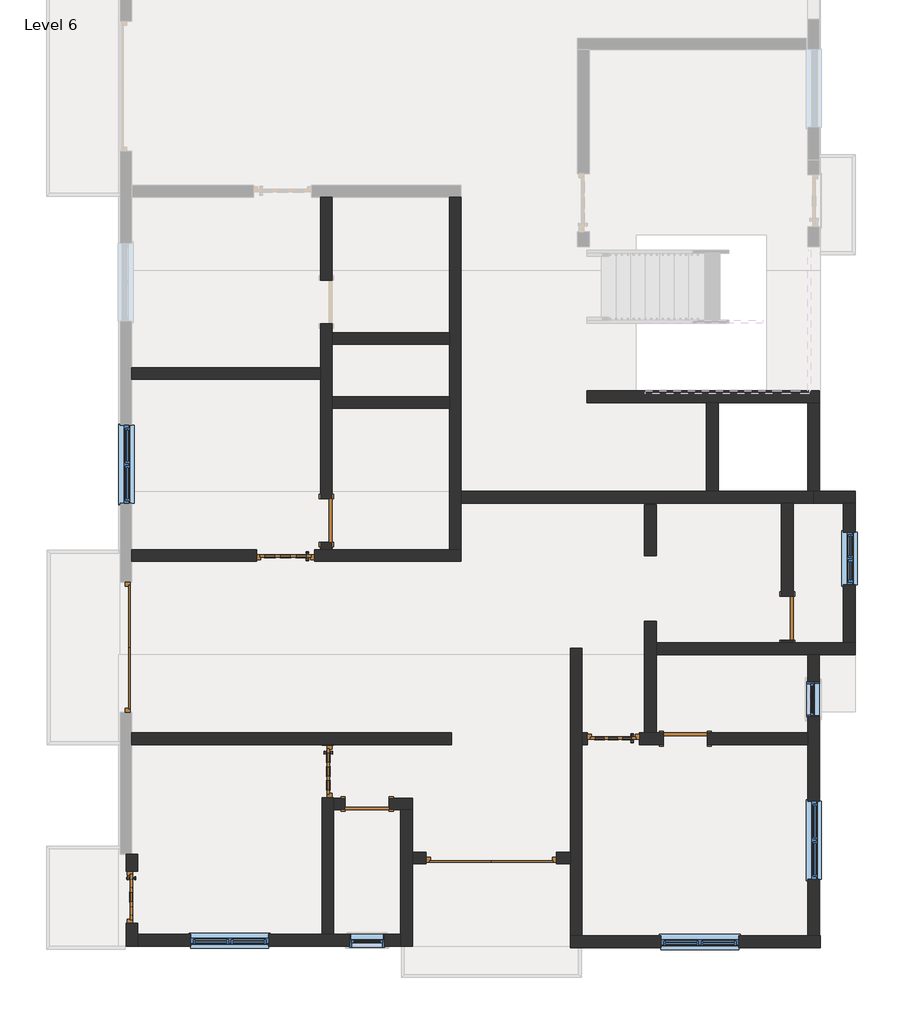
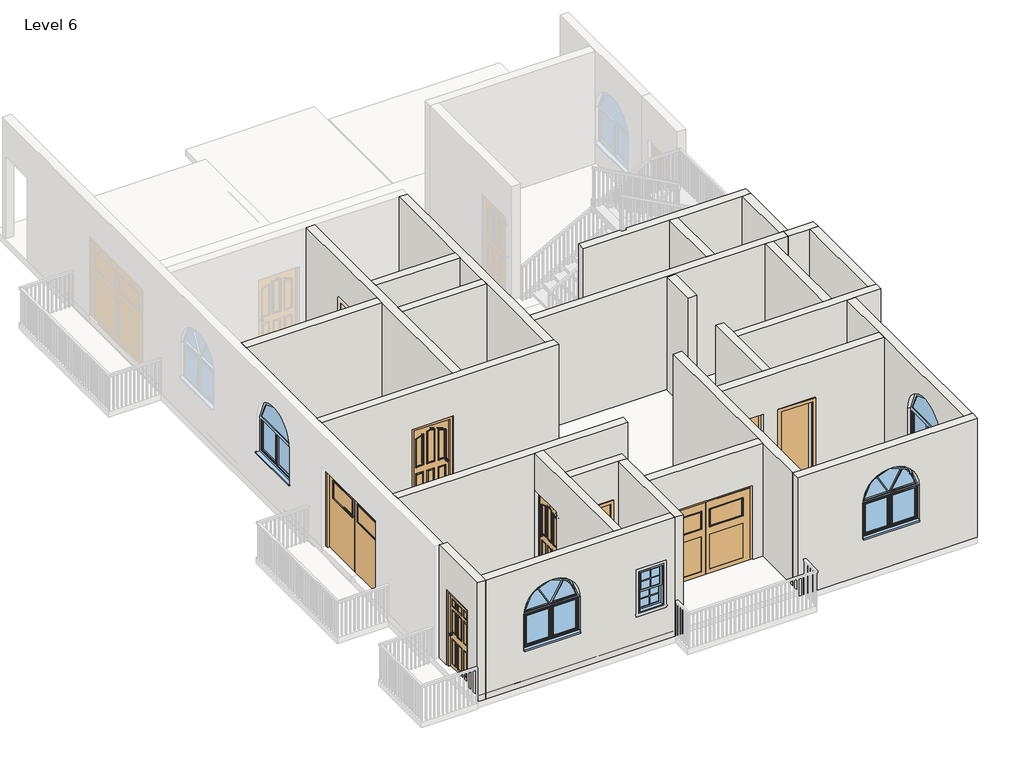
# One storey, part 1 of 7: 27 walls, 10 doors, 7 windows.
# Revit data of these elements (continued)
# Type "Single-Flush : 30\" x 80\"" (continued)
#   Construction Type Id = "MDOOR"
#   Assembly Code = "C1020"
#   Analytic Construction = "Metal"
#   Thickness = 0' - 2"
#   Heat Transfer Coefficient (U) = 0.651978 BTU/(h·ft²·°F)
#   Height = 6' - 8"
#   Trim Projection Ext = 0' - 1"
#   Trim Projection Int = 0' - 1"
#   Trim Width = 0' - 3"
#   Width = 2' - 6"
#   Define Thermal Properties by = 1
#   Define Thermal Properties by = 1
#   Door Material = Door - Panel
#   Frame Material = Door - Frame
#   Visual Light Transmittance = 0
#   Solar Heat Gain Coefficient = 0
#   Function = (empty or 0)
#   Wall Closure = (empty or 0)
# Type "Generic - 9\" w"
#   Assembly Code = "B2010"
#   Layers, outside or top first: 0' - 8" no material (function 1)
# Type "Generic -4.5\" p"
#   Assembly Code = "B2010"
#   Layers, outside or top first: 0' - 8" no material (function 1)
# Type "Window-Double-Hung : 24\" x 42\""
#   Type Mark = "10"
#   Fire Rating = "0.5h"
#   Construction Type Id = "DG-DR"
#   Assembly Code = "B2020100"
#   Analytic Construction = "Double glazing - domestic"
#   Wall Thickness [instance default] = 0' - 6"
#   Window Inset [instance default] = 0' - 0"
#   Visual Light Transmittance = 0.81
#   Thermal Resistance (R) = 1.8146 (h·ft²·°F)/BTU
#   Solar Heat Gain Coefficient = 0.76
#   Muntin Width = 1' - 6"
#   Muntin Height = 1' - 5 1/8"
#   Interior Wall Closure [instance default] = 0' - 1 1/2"
#   Rough Width = 2' - 0 1/2"
#   Rough Height = 3' - 6 1/2"
#   Frame Extension [instance default] = 0' - 1 1/4"
#   Exterior Wall Closure [instance default] = 0' - 0 1/2"
#   Extension Jamb [instance default] = 0' - 1 1/2"
#   Heat Transfer Coefficient (U) = 0.5511 BTU/(h·ft²·°F)
#   Height = 3' - 6"
#   Width = 2' - 0"
#   Define Thermal Properties by = 1
#   Top Muntin Visibility = yes
#   Indicator Visibility [instance default] = yes
#   Extension Jamb Visibility [instance default] = yes
#   Interior Trim Visibility [instance default] = yes
#   Exterior Trim Visibility [instance default] = yes
#   Define Thermal Properties by = 1
#   Bottom Muntin Visibility = yes
#   Muntin Pattern = Muntin Pattern_2x2 : Muntin Pattern_2x2
#   Interior Trim Material = Wood - Stained
#   Interior Trim = Trim-Window-Interior-Flat : Picture Frame
#   Exterior Trim Material = Clad - White
#   Exterior Trim = Trim-Window-Exterior-Flat : with Sill
#   Glass Panel Material = Glass
#   Exterior Frame Material = Clad - White
#   Interior Frame Material = Wood - Stained
#   Wall Closure = (empty or 0)
# Type "Windows_Arched : 1360x910mm"
#   Type Mark = "20"
#   Operation = "UserDefined"
#   Construction Type Id = "GSP4R"
#   Manufacturer = "Revit"
#   Keynote = "L10"
#   Analytic Construction = "1/8 in Pilkington single glazing"
#   Wrap Layers (Ext) from Ext = 0' - 4.03543"
#   Wrap Layers (Int) from Ext = 0' - 6.98819"
#   Window Board Projection = 0' - 0.98425"
#   Window Board Extension = 0' - 0.98425"
#   Visual Light Transmittance = 0.9
#   Solar Heat Gain Coefficient = 0.78
#   Rough Width = 4' - 5.54331"
#   Rough Height = 2' - 11.82677"
#   Height = 2' - 11.82677"
#   Width = 4' - 5.54331"
#   Heat Transfer Coefficient (U) = 0.6496 BTU/(h·ft²·°F)
#   Glazing Thickness = 0' - 0.94488"
#   FrameOffset - External = 0' - 1.9685"
#   Frame Depth = 0' - 2.67717"
#   Default Head Height = 6' - 11.07087"
#   Cill Depth = 0' - 3.44488"
#   Cavity Closer Width = 0' - 1.9685"
#   Cavity Closer Offset from Ext = 0' - 4.03543"
#   Cavity Closer Depth = 0' - 3.34646"
#   Vis - Cavity Closers = yes
#   Define Thermal Properties by = 1
#   Material Trim = Window Frame
#   Material Glass = Glass
#   Material Frame = Window Frame
#   Wall Closure = (empty or 0)
# Type "Windows_Dbl_w-Glazing_Bars : 910x910mm"
#   Type Mark = "33"
#   Operation = "DoublePanelVertical"
#   Construction Type Id = "GSP4R"
#   Manufacturer = "Revit"
#   Keynote = "L10"
#   Analytic Construction = "1/8 in Pilkington single glazing"
#   Wrap Layers (Ext) from Ext = 0' - 4.03543"
#   Wrap Layers (Int) from Ext = 0' - 6.98819"
#   Window Board Projection = 0' - 0.98425"
#   Window Board Extension = 0' - 0.98425"
#   Visual Light Transmittance = 0.9
#   Solar Heat Gain Coefficient = 0.78
#   Rough Width = 2' - 11.82677"
#   Rough Height = 2' - 11.82677"
#   Height = 2' - 11.82677"
#   Width = 2' - 11.82677"
#   Heat Transfer Coefficient (U) = 0.6496 BTU/(h·ft²·°F)
#   Glazing Thickness = 0' - 0.94488"
#   Glazing Bar Thickness = 0' - 0.7874"
#   FrameOffset - External = 0' - 1.9685"
#   Frame Depth = 0' - 2.55906"
#   Default Head Height = 6' - 10.67717"
#   Cill Depth = 0' - 3.44488"
#   Cavity Closer Width = 0' - 1.9685"
#   Cavity Closer Offset from Ext = 0' - 4.03543"
#   Cavity Closer Depth = 0' - 3.34646"
#   Vis - Glazing Bars = yes
#   Vis - Cavity Closers = yes
#   Define Thermal Properties by = 1
#   Material Trim = Window Frame
#   Material Glazing Bars = Window Frame
#   Material Glass = Glass
#   Material Frame = Window Frame
#   Wall Closure = (empty or 0)
# Element 1 (IfcDoor, "Doors_ExtSgl_5 : 910x2110mm")
#   Phase Created = New Construction
#   Materials on its faces: "Door - Panel", "Door - Handle", "Door - Frame/Mullion", "Door - Glazing"
# Element 2 (IfcDoor, "Doors_ExtSgl_6 : 1010x2110mm")
#   Phase Created = New Construction
#   Materials on its faces: "Door - Panel", "Door - Handle", "Door - Frame/Mullion", "Door - Glazing"
# Elements 3, 4 (IfcDoor, "Doors_ExtSgl_6 : 910x2110mm")
#   Phase Created = New Construction
#   Materials on its faces: "Door - Panel", "Door - Handle", "Door - Frame/Mullion", "Door - Glazing"
# Element 5 (IfcDoor, "Doors_Garage_Timber_Side_Hung_Glazing : 2270x2050mm")
#   Phase Created = New Construction
#   Materials on its faces: "Door - Panel", "Door - Frame/Mullion", "Door - Glazing"
# Element 6 (IfcDoor, "Doors_Garage_Timber_Side_Hung_Glazing : 2270x2200mm")
#   Phase Created = New Construction
#   Materials on its faces: "Door - Panel", "Door - Frame/Mullion", "Door - Glazing"
# Elements 7, 8, 9, 10 (IfcDoor, "Single-Flush : 30\" x 80\"")
#   Phase Created = New Construction
#   Materials on its faces: "Door - Frame", "Door - Panel"
# Elements 11, 17 (IfcWall, "Generic - 9\" w")
#   Top Offset = 0' - 0"
#   Base Offset = 0' - 0"
#   wall height = 10' - 0"
#   Phase Created = New Construction
#   Base Constraint = Level 6
#   Top Constraint = Level 7
#   Materials on its faces: "Default Wall", "Earth"
# Elements 12, 13 (IfcWall, "Generic - 9\" w")
#   Top Offset = 0' - 0"
#   Base Offset = 0' - 0"
#   wall height = 10' - 0"
#   Phase Created = New Construction
#   Base Constraint = Level 6
#   Top Constraint = Level 7
#   Materials on its faces: "Default Wall"
# Element 14 (IfcWall, "Generic - 9\" w")
#   Top Offset = 0' - 0"
#   Base Offset = 0' - 0"
#   wall height = 10' - 0"
#   Phase Created = New Construction
#   Base Constraint = Level 6
#   Top Constraint = Level 7
#   Materials on its faces: "Default Wall", "Door - Frame/Mullion", "Earth"
# Element 15 (IfcWall, "Generic - 9\" w")
#   Top Offset = 0' - 0"
#   Base Offset = 0' - 0"
#   wall height = 10' - 0"
#   Phase Created = New Construction
#   Base Constraint = Level 6
#   Top Constraint = Level 7
#   Materials on its faces: "Default Wall", "Concrete, Lightweight", "Wood - Stained"
# Element 16 (IfcWall, "Generic - 9\" w")
#   Top Offset = 0' - 0"
#   Base Offset = 0' - 0"
#   wall height = 10' - 0"
#   Phase Created = New Construction
#   Base Constraint = Level 6
#   Top Constraint = Level 7
#   Materials on its faces: "Default Wall", "Wood - Stained"
# Elements 18, 19 (IfcWall, "Generic - 9\" w")
#   Top Offset = 0' - 0"
#   Base Offset = 0' - 0"
#   wall height = 10' - 0"
#   Phase Created = New Construction
#   Base Constraint = Level 6
#   Top Constraint = Level 7
#   Materials on its faces: "Default Wall", "Concrete, Lightweight"
# Elements 20, 21, 22, 23, 24, 25, 26, 27, 28, 31, 32, 33, 36, 37 (IfcWall, "Generic -4.5\" p")
#   Top Offset = 0' - 0"
#   Base Offset = 0' - 0"
#   wall height = 10' - 0"
#   Phase Created = New Construction
#   Base Constraint = Level 6
#   Top Constraint = Level 7
#   Materials on its faces: "Default Wall"
# Element 29 (IfcWall, "Generic -4.5\" p")
#   Top Offset = 0' - 0"
#   Base Offset = 0' - 0"
#   wall height = 10' - 0"
#   Phase Created = New Construction
#   Base Constraint = Level 6
#   Top Constraint = Level 7
#   Materials on its faces: "Default Wall", "Concrete, Lightweight"
# Element 30 (IfcWall, "Generic -4.5\" p")
#   Top Offset = 0' - 0"
#   Base Offset = 0' - 0"
#   wall height = 10' - 0"
#   Phase Created = New Construction
#   Base Constraint = Level 6
#   Top Constraint = Level 7
#   Materials on its faces: "Default Wall", "Door - Frame/Mullion"
# Elements 34, 35 (IfcWall, "Generic -4.5\" p")
#   Top Offset = 0' - 0"
#   Base Offset = 0' - 0"
#   wall height = 10' - 0"
#   Phase Created = New Construction
#   Base Constraint = Level 6
#   Top Constraint = Level 7
#   Materials on its faces: "Default Wall", "Earth"
# Element 38 (IfcWindow, "Window-Double-Hung : 24\" x 42\"")
#   Mark = "73"
#   Window Inset = 0' - 0"
#   Interior Wall Closure = 0' - 1 1/2"
#   Frame Extension = 0' - 1 1/4"
#   Exterior Wall Closure = 0' - 0 1/2"
#   Interior Trim Visibility = yes
#   Indicator Visibility = yes
#   Exterior Trim Visibility = yes
#   Phase Created = New Construction
#   Materials on its faces: "Wood - Stained", "Glass", "Clad - White"
# Element 39 (IfcWindow, "Window-Double-Hung : 24\" x 42\"")
#   Mark = "92"
#   Window Inset = 0' - 0"
#   Interior Wall Closure = 0' - 1 1/2"
#   Frame Extension = 0' - 1 1/4"
#   Exterior Wall Closure = 0' - 0 1/2"
#   Interior Trim Visibility = yes
#   Indicator Visibility = yes
#   Exterior Trim Visibility = yes
#   Phase Created = New Construction
#   Materials on its faces: "Wood - Stained", "Glass", "Clad - White"
# Element 40 (IfcWindow, "Windows_Arched : 1360x910mm")
#   Mark = "69"
#   Phase Created = New Construction
#   Materials on its faces: "Window Frame", "Glass"
# Element 41 (IfcWindow, "Windows_Arched : 1360x910mm")
#   Mark = "70"
#   Phase Created = New Construction
#   Materials on its faces: "Window Frame", "Glass"
# Element 42 (IfcWindow, "Windows_Arched : 1360x910mm")
#   Mark = "71"
#   Phase Created = New Construction
#   Materials on its faces: "Window Frame", "Glass"
# Element 43 (IfcWindow, "Windows_Arched : 1360x910mm")
#   Mark = "87"
#   Phase Created = New Construction
#   Materials on its faces: "Window Frame", "Glass"
# Element 44 (IfcWindow, "Windows_Dbl_w-Glazing_Bars : 910x910mm")
#   Mark = "74"
#   Phase Created = New Construction
#   Materials on its faces: "Window Frame", "Glass"
# Materials
#   "Door - Glazing": colour RGB 0 0 255, transparency 0.75
#   "Door - Panel": class "Wood", colour RGB 210 159 95, transparency 0, Cost = 0
#   "Door - Frame/Mullion": class "Wood", colour RGB 212 179 113, transparency 0
#   "Door - Handle": colour RGB 0 0 0, transparency 0
#   "Door - Frame": colour RGB 118 70 51, transparency 0, Cost = 0
#   "Wood - Stained": class "Wood", colour RGB 224 178 126, transparency 0, Cost = 0
#   "Clad - White": class "Wood", colour RGB 242 242 238, transparency 0, Cost = 0
#   "Glass": class "Glass", colour RGB 0 128 192, transparency 0.75, Description = "Soda Lime Glass", Cost = 0
#   "Window Frame": colour RGB 249 249 249, transparency 0
#   "Default Wall": colour RGB 128 128 128, transparency 0, Cost = 0
#   "Earth": class "Generic", colour RGB 97 75 62, transparency 0, Description = "Soil", Cost = 0
#   "Concrete, Lightweight": class "Concrete", colour RGB 142 141 140, transparency 0, Description = "Lightweight concrete", Cost = 0
